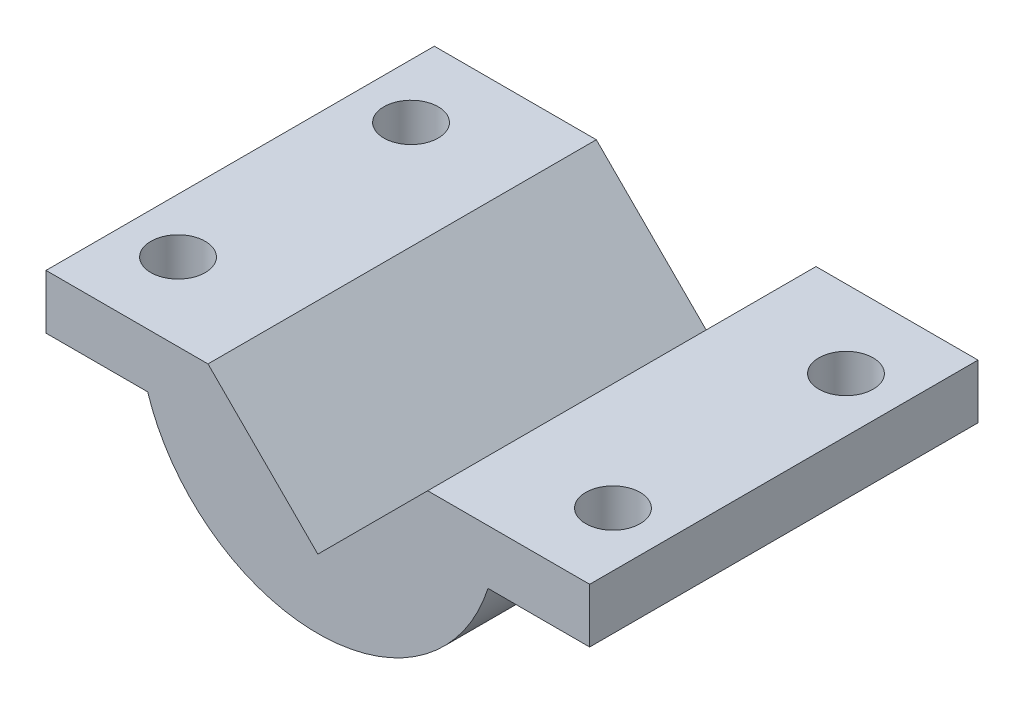
ISO-10303-21;
HEADER;
FILE_DESCRIPTION(('STEP AP214'),'2;1');
FILE_NAME('part.step','',(''),(''),'','','');
FILE_SCHEMA(('AUTOMOTIVE_DESIGN { 1 0 10303 214 1 1 1 1 }'));
ENDSEC;
DATA;
#1=APPLICATION_CONTEXT('core data for automotive mechanical design processes');
#2=APPLICATION_PROTOCOL_DEFINITION('international standard','automotive_design',2000,#1);
#3=PRODUCT_CONTEXT('',#1,'mechanical');
#4=PRODUCT('Part','Part','',(#3));
#5=PRODUCT_RELATED_PRODUCT_CATEGORY('part','',(#4));
#6=PRODUCT_DEFINITION_FORMATION('','',#4);
#7=PRODUCT_DEFINITION_CONTEXT('part definition',#1,'design');
#8=PRODUCT_DEFINITION('design','',#6,#7);
#9=PRODUCT_DEFINITION_SHAPE('','',#8);
#10=(LENGTH_UNIT() NAMED_UNIT(*) SI_UNIT(.MILLI.,.METRE.));
#11=(NAMED_UNIT(*) PLANE_ANGLE_UNIT() SI_UNIT($,.RADIAN.));
#12=(NAMED_UNIT(*) SI_UNIT($,.STERADIAN.) SOLID_ANGLE_UNIT());
#13=UNCERTAINTY_MEASURE_WITH_UNIT(LENGTH_MEASURE(1.E-05),#10,'distance_accuracy_value','');
#14=(GEOMETRIC_REPRESENTATION_CONTEXT(3) GLOBAL_UNCERTAINTY_ASSIGNED_CONTEXT((#13)) GLOBAL_UNIT_ASSIGNED_CONTEXT((#10,
#11,#12)) REPRESENTATION_CONTEXT('',''));
#15=CARTESIAN_POINT('',(0.,0.,0.));
#16=DIRECTION('',(0.,0.,1.));
#17=DIRECTION('',(1.,0.,0.));
#18=AXIS2_PLACEMENT_3D('',#15,#16,#17);
#19=CARTESIAN_POINT('',(-14.142135623731,0.,25.));
#20=DIRECTION('',(0.,-1.,0.));
#21=DIRECTION('',(1.,0.,0.));
#22=AXIS2_PLACEMENT_3D('',#19,#20,#21);
#23=PLANE('',#22);
#24=CARTESIAN_POINT('',(-28.,0.,15.));
#25=DIRECTION('',(0.,1.,0.));
#26=DIRECTION('',(-1.,0.,0.));
#27=AXIS2_PLACEMENT_3D('',#24,#25,#26);
#28=CIRCLE('',#27,3.5);
#29=CARTESIAN_POINT('',(-31.5,0.,15.));
#30=VERTEX_POINT('',#29);
#31=EDGE_CURVE('E214',#30,#30,#28,.T.);
#32=ORIENTED_EDGE('',*,*,#31,.F.);
#33=EDGE_LOOP('',(#32));
#34=FACE_BOUND('',#33,.T.);
#35=CARTESIAN_POINT('',(-28.,0.,-15.));
#36=DIRECTION('',(0.,1.,0.));
#37=DIRECTION('',(-1.,0.,0.));
#38=AXIS2_PLACEMENT_3D('',#35,#36,#37);
#39=CIRCLE('',#38,3.5);
#40=CARTESIAN_POINT('',(-31.5,0.,-15.));
#41=VERTEX_POINT('',#40);
#42=EDGE_CURVE('E203',#41,#41,#39,.T.);
#43=ORIENTED_EDGE('',*,*,#42,.F.);
#44=EDGE_LOOP('',(#43));
#45=FACE_BOUND('',#44,.T.);
#46=DIRECTION('',(-1.,0.,0.));
#47=VECTOR('',#46,1.);
#48=CARTESIAN_POINT('',(-14.142135623731,0.,-25.));
#49=LINE('',#48,#47);
#50=CARTESIAN_POINT('',(-14.142135623731,0.,-25.));
#51=VERTEX_POINT('',#50);
#52=CARTESIAN_POINT('',(-35.,0.,-25.));
#53=VERTEX_POINT('',#52);
#54=EDGE_CURVE('E143',#51,#53,#49,.T.);
#55=ORIENTED_EDGE('',*,*,#54,.T.);
#56=DIRECTION('',(0.,0.,-1.));
#57=VECTOR('',#56,1.);
#58=CARTESIAN_POINT('',(-35.,0.,25.));
#59=LINE('',#58,#57);
#60=CARTESIAN_POINT('',(-35.,0.,25.));
#61=VERTEX_POINT('',#60);
#62=EDGE_CURVE('E11',#61,#53,#59,.T.);
#63=ORIENTED_EDGE('',*,*,#62,.F.);
#64=DIRECTION('',(-1.,0.,0.));
#65=VECTOR('',#64,1.);
#66=CARTESIAN_POINT('',(-14.142135623731,0.,25.));
#67=LINE('',#66,#65);
#68=CARTESIAN_POINT('',(-14.142135623731,0.,25.));
#69=VERTEX_POINT('',#68);
#70=EDGE_CURVE('E158',#69,#61,#67,.T.);
#71=ORIENTED_EDGE('',*,*,#70,.F.);
#72=DIRECTION('',(0.,0.,-1.));
#73=VECTOR('',#72,1.);
#74=CARTESIAN_POINT('',(-14.142135623731,0.,25.));
#75=LINE('',#74,#73);
#76=EDGE_CURVE('E140',#69,#51,#75,.T.);
#77=ORIENTED_EDGE('',*,*,#76,.T.);
#78=EDGE_LOOP('',(#55,#63,#71,#77));
#79=FACE_BOUND('',#78,.T.);
#80=ADVANCED_FACE('F39',(#34,#45,#79),#23,.F.);
#81=CARTESIAN_POINT('',(-35.,0.,25.));
#82=DIRECTION('',(1.,0.,0.));
#83=DIRECTION('',(0.,0.,-1.));
#84=AXIS2_PLACEMENT_3D('',#81,#82,#83);
#85=PLANE('',#84);
#86=DIRECTION('',(0.,-1.,0.));
#87=VECTOR('',#86,1.);
#88=CARTESIAN_POINT('',(-35.,0.,-25.));
#89=LINE('',#88,#87);
#90=CARTESIAN_POINT('',(-35.,-7.,-25.));
#91=VERTEX_POINT('',#90);
#92=EDGE_CURVE('E145',#53,#91,#89,.T.);
#93=ORIENTED_EDGE('',*,*,#92,.T.);
#94=DIRECTION('',(0.,0.,-1.));
#95=VECTOR('',#94,1.);
#96=CARTESIAN_POINT('',(-35.,-7.,25.));
#97=LINE('',#96,#95);
#98=CARTESIAN_POINT('',(-35.,-7.,25.));
#99=VERTEX_POINT('',#98);
#100=EDGE_CURVE('E50',#99,#91,#97,.T.);
#101=ORIENTED_EDGE('',*,*,#100,.F.);
#102=DIRECTION('',(0.,-1.,0.));
#103=VECTOR('',#102,1.);
#104=CARTESIAN_POINT('',(-35.,0.,25.));
#105=LINE('',#104,#103);
#106=EDGE_CURVE('E101',#61,#99,#105,.T.);
#107=ORIENTED_EDGE('',*,*,#106,.F.);
#108=ORIENTED_EDGE('',*,*,#62,.T.);
#109=EDGE_LOOP('',(#93,#101,#107,#108));
#110=FACE_BOUND('',#109,.T.);
#111=ADVANCED_FACE('F229',(#110),#85,.F.);
#112=CARTESIAN_POINT('',(-35.,-7.,25.));
#113=DIRECTION('',(0.,1.,0.));
#114=DIRECTION('',(-1.,0.,0.));
#115=AXIS2_PLACEMENT_3D('',#112,#113,#114);
#116=PLANE('',#115);
#117=CARTESIAN_POINT('',(-28.,-7.,15.));
#118=DIRECTION('',(0.,1.,0.));
#119=DIRECTION('',(-1.,0.,0.));
#120=AXIS2_PLACEMENT_3D('',#117,#118,#119);
#121=CIRCLE('',#120,3.5);
#122=CARTESIAN_POINT('',(-31.5,-7.,15.));
#123=VERTEX_POINT('',#122);
#124=EDGE_CURVE('E204',#123,#123,#121,.F.);
#125=ORIENTED_EDGE('',*,*,#124,.F.);
#126=EDGE_LOOP('',(#125));
#127=FACE_BOUND('',#126,.T.);
#128=CARTESIAN_POINT('',(-28.,-7.,-15.));
#129=DIRECTION('',(0.,1.,0.));
#130=DIRECTION('',(-1.,0.,0.));
#131=AXIS2_PLACEMENT_3D('',#128,#129,#130);
#132=CIRCLE('',#131,3.5);
#133=CARTESIAN_POINT('',(-31.5,-7.,-15.));
#134=VERTEX_POINT('',#133);
#135=EDGE_CURVE('E144',#134,#134,#132,.F.);
#136=ORIENTED_EDGE('',*,*,#135,.F.);
#137=EDGE_LOOP('',(#136));
#138=FACE_BOUND('',#137,.T.);
#139=DIRECTION('',(1.,0.,0.));
#140=VECTOR('',#139,1.);
#141=CARTESIAN_POINT('',(-35.,-7.,-25.));
#142=LINE('',#141,#140);
#143=CARTESIAN_POINT('',(-21.9089023002066,-7.,-25.));
#144=VERTEX_POINT('',#143);
#145=EDGE_CURVE('E150',#91,#144,#142,.T.);
#146=ORIENTED_EDGE('',*,*,#145,.T.);
#147=DIRECTION('',(0.,0.,-1.));
#148=VECTOR('',#147,1.);
#149=CARTESIAN_POINT('',(-21.9089023002066,-7.,25.));
#150=LINE('',#149,#148);
#151=CARTESIAN_POINT('',(-21.9089023002066,-7.,25.));
#152=VERTEX_POINT('',#151);
#153=EDGE_CURVE('E169',#152,#144,#150,.T.);
#154=ORIENTED_EDGE('',*,*,#153,.F.);
#155=DIRECTION('',(1.,0.,0.));
#156=VECTOR('',#155,1.);
#157=CARTESIAN_POINT('',(-35.,-7.,25.));
#158=LINE('',#157,#156);
#159=EDGE_CURVE('E178',#99,#152,#158,.T.);
#160=ORIENTED_EDGE('',*,*,#159,.F.);
#161=ORIENTED_EDGE('',*,*,#100,.T.);
#162=EDGE_LOOP('',(#146,#154,#160,#161));
#163=FACE_BOUND('',#162,.T.);
#164=ADVANCED_FACE('F171',(#127,#138,#163),#116,.F.);
#165=CARTESIAN_POINT('',(0.,0.,25.));
#166=DIRECTION('',(0.,0.,-1.));
#167=DIRECTION('',(-1.,0.,0.));
#168=AXIS2_PLACEMENT_3D('',#165,#166,#167);
#169=CYLINDRICAL_SURFACE('',#168,23.);
#170=CARTESIAN_POINT('',(0.,0.,-25.));
#171=DIRECTION('',(0.,0.,1.));
#172=DIRECTION('',(1.,0.,0.));
#173=AXIS2_PLACEMENT_3D('',#170,#171,#172);
#174=CIRCLE('',#173,23.);
#175=CARTESIAN_POINT('',(21.9089023002066,-7.,-25.));
#176=VERTEX_POINT('',#175);
#177=EDGE_CURVE('E149',#144,#176,#174,.T.);
#178=ORIENTED_EDGE('',*,*,#177,.T.);
#179=DIRECTION('',(0.,0.,-1.));
#180=VECTOR('',#179,1.);
#181=CARTESIAN_POINT('',(21.9089023002066,-7.,25.));
#182=LINE('',#181,#180);
#183=CARTESIAN_POINT('',(21.9089023002066,-7.,25.));
#184=VERTEX_POINT('',#183);
#185=EDGE_CURVE('E164',#184,#176,#182,.T.);
#186=ORIENTED_EDGE('',*,*,#185,.F.);
#187=CARTESIAN_POINT('',(0.,0.,25.));
#188=DIRECTION('',(0.,0.,1.));
#189=DIRECTION('',(1.,0.,0.));
#190=AXIS2_PLACEMENT_3D('',#187,#188,#189);
#191=CIRCLE('',#190,23.);
#192=EDGE_CURVE('E195',#152,#184,#191,.T.);
#193=ORIENTED_EDGE('',*,*,#192,.F.);
#194=ORIENTED_EDGE('',*,*,#153,.T.);
#195=EDGE_LOOP('',(#178,#186,#193,#194));
#196=FACE_BOUND('',#195,.T.);
#197=ADVANCED_FACE('F183',(#196),#169,.T.);
#198=CARTESIAN_POINT('',(35.,-6.99999999999999,25.));
#199=DIRECTION('',(0.,1.,0.));
#200=DIRECTION('',(-1.,0.,0.));
#201=AXIS2_PLACEMENT_3D('',#198,#199,#200);
#202=PLANE('',#201);
#203=CARTESIAN_POINT('',(28.,-7.,-15.));
#204=DIRECTION('',(0.,1.,0.));
#205=DIRECTION('',(-1.,0.,0.));
#206=AXIS2_PLACEMENT_3D('',#203,#204,#205);
#207=CIRCLE('',#206,3.5);
#208=CARTESIAN_POINT('',(24.5,-7.,-15.));
#209=VERTEX_POINT('',#208);
#210=EDGE_CURVE('E202',#209,#209,#207,.F.);
#211=ORIENTED_EDGE('',*,*,#210,.F.);
#212=EDGE_LOOP('',(#211));
#213=FACE_BOUND('',#212,.T.);
#214=CARTESIAN_POINT('',(28.,-7.,15.));
#215=DIRECTION('',(0.,1.,0.));
#216=DIRECTION('',(-1.,0.,0.));
#217=AXIS2_PLACEMENT_3D('',#214,#215,#216);
#218=CIRCLE('',#217,3.5);
#219=CARTESIAN_POINT('',(24.5,-7.,15.));
#220=VERTEX_POINT('',#219);
#221=EDGE_CURVE('E215',#220,#220,#218,.F.);
#222=ORIENTED_EDGE('',*,*,#221,.F.);
#223=EDGE_LOOP('',(#222));
#224=FACE_BOUND('',#223,.T.);
#225=DIRECTION('',(1.,0.,0.));
#226=VECTOR('',#225,1.);
#227=CARTESIAN_POINT('',(35.,-6.99999999999999,-25.));
#228=LINE('',#227,#226);
#229=CARTESIAN_POINT('',(35.,-6.99999999999999,-25.));
#230=VERTEX_POINT('',#229);
#231=EDGE_CURVE('E151',#176,#230,#228,.T.);
#232=ORIENTED_EDGE('',*,*,#231,.T.);
#233=DIRECTION('',(0.,0.,-1.));
#234=VECTOR('',#233,1.);
#235=CARTESIAN_POINT('',(35.,-6.99999999999999,25.));
#236=LINE('',#235,#234);
#237=CARTESIAN_POINT('',(35.,-6.99999999999999,25.));
#238=VERTEX_POINT('',#237);
#239=EDGE_CURVE('E165',#238,#230,#236,.T.);
#240=ORIENTED_EDGE('',*,*,#239,.F.);
#241=DIRECTION('',(1.,0.,0.));
#242=VECTOR('',#241,1.);
#243=CARTESIAN_POINT('',(35.,-6.99999999999999,25.));
#244=LINE('',#243,#242);
#245=EDGE_CURVE('E193',#184,#238,#244,.T.);
#246=ORIENTED_EDGE('',*,*,#245,.F.);
#247=ORIENTED_EDGE('',*,*,#185,.T.);
#248=EDGE_LOOP('',(#232,#240,#246,#247));
#249=FACE_BOUND('',#248,.T.);
#250=ADVANCED_FACE('F186',(#213,#224,#249),#202,.F.);
#251=CARTESIAN_POINT('',(35.,0.,25.));
#252=DIRECTION('',(-1.,0.,0.));
#253=DIRECTION('',(0.,-1.,0.));
#254=AXIS2_PLACEMENT_3D('',#251,#252,#253);
#255=PLANE('',#254);
#256=DIRECTION('',(0.,1.,0.));
#257=VECTOR('',#256,1.);
#258=CARTESIAN_POINT('',(35.,0.,-25.));
#259=LINE('',#258,#257);
#260=CARTESIAN_POINT('',(35.,0.,-25.));
#261=VERTEX_POINT('',#260);
#262=EDGE_CURVE('E153',#230,#261,#259,.T.);
#263=ORIENTED_EDGE('',*,*,#262,.T.);
#264=DIRECTION('',(0.,0.,-1.));
#265=VECTOR('',#264,1.);
#266=CARTESIAN_POINT('',(35.,0.,25.));
#267=LINE('',#266,#265);
#268=CARTESIAN_POINT('',(35.,0.,25.));
#269=VERTEX_POINT('',#268);
#270=EDGE_CURVE('E135',#269,#261,#267,.T.);
#271=ORIENTED_EDGE('',*,*,#270,.F.);
#272=DIRECTION('',(0.,1.,0.));
#273=VECTOR('',#272,1.);
#274=CARTESIAN_POINT('',(35.,0.,25.));
#275=LINE('',#274,#273);
#276=EDGE_CURVE('E121',#238,#269,#275,.T.);
#277=ORIENTED_EDGE('',*,*,#276,.F.);
#278=ORIENTED_EDGE('',*,*,#239,.T.);
#279=EDGE_LOOP('',(#263,#271,#277,#278));
#280=FACE_BOUND('',#279,.T.);
#281=ADVANCED_FACE('F232',(#280),#255,.F.);
#282=CARTESIAN_POINT('',(14.142135623731,0.,25.));
#283=DIRECTION('',(0.,-1.,0.));
#284=DIRECTION('',(1.,0.,0.));
#285=AXIS2_PLACEMENT_3D('',#282,#283,#284);
#286=PLANE('',#285);
#287=CARTESIAN_POINT('',(28.,0.,-15.));
#288=DIRECTION('',(0.,1.,0.));
#289=DIRECTION('',(1.,0.,0.));
#290=AXIS2_PLACEMENT_3D('',#287,#288,#289);
#291=CIRCLE('',#290,3.5);
#292=CARTESIAN_POINT('',(31.5,0.,-15.));
#293=VERTEX_POINT('',#292);
#294=EDGE_CURVE('E207',#293,#293,#291,.T.);
#295=ORIENTED_EDGE('',*,*,#294,.F.);
#296=EDGE_LOOP('',(#295));
#297=FACE_BOUND('',#296,.T.);
#298=CARTESIAN_POINT('',(28.,0.,15.));
#299=DIRECTION('',(0.,1.,0.));
#300=DIRECTION('',(1.,0.,0.));
#301=AXIS2_PLACEMENT_3D('',#298,#299,#300);
#302=CIRCLE('',#301,3.5);
#303=CARTESIAN_POINT('',(31.5,0.,15.));
#304=VERTEX_POINT('',#303);
#305=EDGE_CURVE('E208',#304,#304,#302,.T.);
#306=ORIENTED_EDGE('',*,*,#305,.F.);
#307=EDGE_LOOP('',(#306));
#308=FACE_BOUND('',#307,.T.);
#309=DIRECTION('',(-1.,0.,0.));
#310=VECTOR('',#309,1.);
#311=CARTESIAN_POINT('',(14.142135623731,0.,-25.));
#312=LINE('',#311,#310);
#313=CARTESIAN_POINT('',(14.142135623731,0.,-25.));
#314=VERTEX_POINT('',#313);
#315=EDGE_CURVE('E132',#261,#314,#312,.T.);
#316=ORIENTED_EDGE('',*,*,#315,.T.);
#317=DIRECTION('',(0.,0.,-1.));
#318=VECTOR('',#317,1.);
#319=CARTESIAN_POINT('',(14.142135623731,0.,25.));
#320=LINE('',#319,#318);
#321=CARTESIAN_POINT('',(14.142135623731,0.,25.));
#322=VERTEX_POINT('',#321);
#323=EDGE_CURVE('E126',#322,#314,#320,.T.);
#324=ORIENTED_EDGE('',*,*,#323,.F.);
#325=DIRECTION('',(-1.,0.,0.));
#326=VECTOR('',#325,1.);
#327=CARTESIAN_POINT('',(14.142135623731,0.,25.));
#328=LINE('',#327,#326);
#329=EDGE_CURVE('E120',#269,#322,#328,.T.);
#330=ORIENTED_EDGE('',*,*,#329,.F.);
#331=ORIENTED_EDGE('',*,*,#270,.T.);
#332=EDGE_LOOP('',(#316,#324,#330,#331));
#333=FACE_BOUND('',#332,.T.);
#334=ADVANCED_FACE('F129',(#297,#308,#333),#286,.F.);
#335=CARTESIAN_POINT('',(0.,-14.1421356237308,25.));
#336=DIRECTION('',(0.70710678118654,-0.707106781186555,0.));
#337=DIRECTION('',(0.707106781186555,0.70710678118654,0.));
#338=AXIS2_PLACEMENT_3D('',#335,#336,#337);
#339=PLANE('',#338);
#340=DIRECTION('',(-0.707106781186555,-0.70710678118654,0.));
#341=VECTOR('',#340,1.);
#342=CARTESIAN_POINT('',(0.,-14.1421356237308,-25.));
#343=LINE('',#342,#341);
#344=CARTESIAN_POINT('',(0.,-14.1421356237308,-25.));
#345=VERTEX_POINT('',#344);
#346=EDGE_CURVE('E87',#314,#345,#343,.T.);
#347=ORIENTED_EDGE('',*,*,#346,.T.);
#348=DIRECTION('',(0.,0.,-1.));
#349=VECTOR('',#348,1.);
#350=CARTESIAN_POINT('',(0.,-14.1421356237308,25.));
#351=LINE('',#350,#349);
#352=CARTESIAN_POINT('',(0.,-14.1421356237308,25.));
#353=VERTEX_POINT('',#352);
#354=EDGE_CURVE('E134',#353,#345,#351,.T.);
#355=ORIENTED_EDGE('',*,*,#354,.F.);
#356=DIRECTION('',(-0.707106781186555,-0.70710678118654,0.));
#357=VECTOR('',#356,1.);
#358=CARTESIAN_POINT('',(0.,-14.1421356237308,25.));
#359=LINE('',#358,#357);
#360=EDGE_CURVE('E123',#322,#353,#359,.T.);
#361=ORIENTED_EDGE('',*,*,#360,.F.);
#362=ORIENTED_EDGE('',*,*,#323,.T.);
#363=EDGE_LOOP('',(#347,#355,#361,#362));
#364=FACE_BOUND('',#363,.T.);
#365=ADVANCED_FACE('F133',(#364),#339,.F.);
#366=CARTESIAN_POINT('',(0.,-14.1421356237308,25.));
#367=DIRECTION('',(-0.707106781186544,-0.707106781186551,0.));
#368=DIRECTION('',(0.707106781186551,-0.707106781186544,0.));
#369=AXIS2_PLACEMENT_3D('',#366,#367,#368);
#370=PLANE('',#369);
#371=DIRECTION('',(-0.707106781186551,0.707106781186544,0.));
#372=VECTOR('',#371,1.);
#373=CARTESIAN_POINT('',(0.,-14.1421356237308,-25.));
#374=LINE('',#373,#372);
#375=EDGE_CURVE('E91',#345,#51,#374,.T.);
#376=ORIENTED_EDGE('',*,*,#375,.T.);
#377=ORIENTED_EDGE('',*,*,#76,.F.);
#378=DIRECTION('',(-0.707106781186551,0.707106781186544,0.));
#379=VECTOR('',#378,1.);
#380=CARTESIAN_POINT('',(0.,-14.1421356237308,25.));
#381=LINE('',#380,#379);
#382=EDGE_CURVE('E54',#353,#69,#381,.T.);
#383=ORIENTED_EDGE('',*,*,#382,.F.);
#384=ORIENTED_EDGE('',*,*,#354,.T.);
#385=EDGE_LOOP('',(#376,#377,#383,#384));
#386=FACE_BOUND('',#385,.T.);
#387=ADVANCED_FACE('F292',(#386),#370,.F.);
#388=CARTESIAN_POINT('',(0.,0.,25.));
#389=DIRECTION('',(0.,0.,1.));
#390=DIRECTION('',(1.,0.,0.));
#391=AXIS2_PLACEMENT_3D('',#388,#389,#390);
#392=PLANE('',#391);
#393=ORIENTED_EDGE('',*,*,#70,.T.);
#394=ORIENTED_EDGE('',*,*,#106,.T.);
#395=ORIENTED_EDGE('',*,*,#159,.T.);
#396=ORIENTED_EDGE('',*,*,#192,.T.);
#397=ORIENTED_EDGE('',*,*,#245,.T.);
#398=ORIENTED_EDGE('',*,*,#276,.T.);
#399=ORIENTED_EDGE('',*,*,#329,.T.);
#400=ORIENTED_EDGE('',*,*,#360,.T.);
#401=ORIENTED_EDGE('',*,*,#382,.T.);
#402=EDGE_LOOP('',(#393,#394,#395,#396,#397,#398,#399,#400,#401));
#403=FACE_BOUND('',#402,.T.);
#404=ADVANCED_FACE('F116',(#403),#392,.T.);
#405=CARTESIAN_POINT('',(0.,0.,-25.));
#406=DIRECTION('',(0.,0.,1.));
#407=DIRECTION('',(1.,0.,0.));
#408=AXIS2_PLACEMENT_3D('',#405,#406,#407);
#409=PLANE('',#408);
#410=ORIENTED_EDGE('',*,*,#54,.F.);
#411=ORIENTED_EDGE('',*,*,#375,.F.);
#412=ORIENTED_EDGE('',*,*,#346,.F.);
#413=ORIENTED_EDGE('',*,*,#315,.F.);
#414=ORIENTED_EDGE('',*,*,#262,.F.);
#415=ORIENTED_EDGE('',*,*,#231,.F.);
#416=ORIENTED_EDGE('',*,*,#177,.F.);
#417=ORIENTED_EDGE('',*,*,#145,.F.);
#418=ORIENTED_EDGE('',*,*,#92,.F.);
#419=EDGE_LOOP('',(#410,#411,#412,#413,#414,#415,#416,#417,#418));
#420=FACE_BOUND('',#419,.T.);
#421=ADVANCED_FACE('F179',(#420),#409,.F.);
#422=CARTESIAN_POINT('',(28.,-23.001,15.));
#423=DIRECTION('',(0.,1.,0.));
#424=DIRECTION('',(-1.,0.,0.));
#425=AXIS2_PLACEMENT_3D('',#422,#423,#424);
#426=CYLINDRICAL_SURFACE('',#425,3.5);
#427=ORIENTED_EDGE('',*,*,#305,.T.);
#428=EDGE_LOOP('',(#427));
#429=FACE_BOUND('',#428,.T.);
#430=ORIENTED_EDGE('',*,*,#221,.T.);
#431=EDGE_LOOP('',(#430));
#432=FACE_BOUND('',#431,.T.);
#433=ADVANCED_FACE('F312',(#429,#432),#426,.F.);
#434=CARTESIAN_POINT('',(28.,-23.001,-15.));
#435=DIRECTION('',(0.,1.,0.));
#436=DIRECTION('',(-1.,0.,0.));
#437=AXIS2_PLACEMENT_3D('',#434,#435,#436);
#438=CYLINDRICAL_SURFACE('',#437,3.5);
#439=ORIENTED_EDGE('',*,*,#294,.T.);
#440=EDGE_LOOP('',(#439));
#441=FACE_BOUND('',#440,.T.);
#442=ORIENTED_EDGE('',*,*,#210,.T.);
#443=EDGE_LOOP('',(#442));
#444=FACE_BOUND('',#443,.T.);
#445=ADVANCED_FACE('F323',(#441,#444),#438,.F.);
#446=CARTESIAN_POINT('',(-28.,-23.001,-15.));
#447=DIRECTION('',(0.,1.,0.));
#448=DIRECTION('',(-1.,0.,0.));
#449=AXIS2_PLACEMENT_3D('',#446,#447,#448);
#450=CYLINDRICAL_SURFACE('',#449,3.5);
#451=ORIENTED_EDGE('',*,*,#42,.T.);
#452=EDGE_LOOP('',(#451));
#453=FACE_BOUND('',#452,.T.);
#454=ORIENTED_EDGE('',*,*,#135,.T.);
#455=EDGE_LOOP('',(#454));
#456=FACE_BOUND('',#455,.T.);
#457=ADVANCED_FACE('F334',(#453,#456),#450,.F.);
#458=CARTESIAN_POINT('',(-28.,-23.001,15.));
#459=DIRECTION('',(0.,1.,0.));
#460=DIRECTION('',(-1.,0.,0.));
#461=AXIS2_PLACEMENT_3D('',#458,#459,#460);
#462=CYLINDRICAL_SURFACE('',#461,3.5);
#463=ORIENTED_EDGE('',*,*,#31,.T.);
#464=EDGE_LOOP('',(#463));
#465=FACE_BOUND('',#464,.T.);
#466=ORIENTED_EDGE('',*,*,#124,.T.);
#467=EDGE_LOOP('',(#466));
#468=FACE_BOUND('',#467,.T.);
#469=ADVANCED_FACE('F224',(#465,#468),#462,.F.);
#470=CLOSED_SHELL('',(#80,#111,#164,#197,#250,#281,#334,#365,#387,#404,#421,#433,#445,#457,#469));
#471=MANIFOLD_SOLID_BREP('B2',#470);
#472=ADVANCED_BREP_SHAPE_REPRESENTATION('',(#18,#471),#14);
#473=SHAPE_DEFINITION_REPRESENTATION(#9,#472);
ENDSEC;
END-ISO-10303-21;
